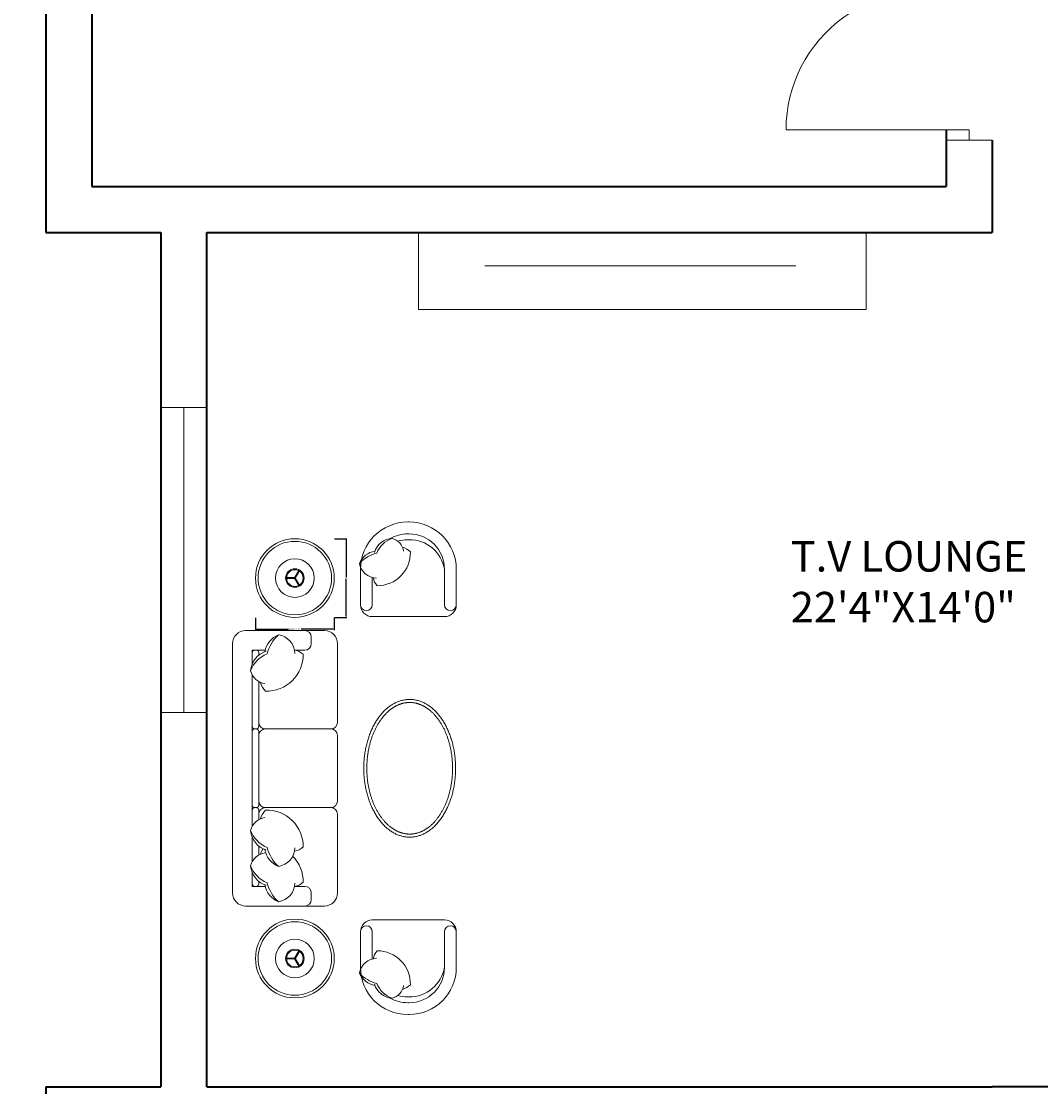
# Model space of a CAD drawing. Units: inches. Extents: x 1824 to 3509, y 619 to 2294.
# Tile 4 of 12: x 2001 to 2202, y 1115 to 1325. Entities that reach past the tile are written whole.
import ezdxf

# ---------------------------------------------------------------- set-up
doc = ezdxf.new("R2010")
doc.units = ezdxf.units.IN
for name, color, linetype, lineweight in [('A-ANNO-DIMS', 2, 'Continuous', 18), ('A-AREA-IDEN', 7, 'Continuous', 18), ('A-DOOR', 3, 'Continuous', 18), ('A-FURN', 8, 'Continuous', 13), ('A-GLAZ', 4, 'Continuous', 18), ('A-WALL', 7, 'Continuous', 35)]:
    doc.layers.add(name, color=color, linetype=linetype, lineweight=lineweight)
doc.styles.get("Standard").update_dxf_attribs({"font": 'arial.ttf'})
doc.dimstyles.get("Standard").update_dxf_attribs({"dimtxt": 0.18, "dimasz": 0.18, "dimexe": 0.18, "dimexo": 0.0625, "dimgap": 0.09, "dimtad": 0, "dimtih": 1, "dimtoh": 1, "dimdec": 4, "dimzin": 0, "dimdsep": 46, "dimtxsty": 'Standard', "dimcen": 0.09, "dimadec": 0, "dimazin": 0, "dimtfac": 1, "dimtdec": 4, "dimtofl": 0, "dimtmove": 0, "dimatfit": 3, "dimfxl": 1, "dimtolj": 1, "dimtzin": 0, "dimarcsym": 0})

# ---------------------------------------------------------------- blocks, each defined once
blk = doc.blocks.new('DOOR-BED-W-36')
for p, q in [((31.5, 29.8), (40.5, 29.8)), ((40.5, 29.8), (36, 29.8)), ((36, 29.8), (36, 27.8)), ((36, 2), (0, 2)), ((31.5, 0), (31.5, 0)), ((31.5, 0), (40.5, 0)), ((36, 0), (36, 2)), ((40.5, 0), (36, 0)), ((36, 0), (36, 0)), ((40.5, 0), (40.5, 0))]:
    blk.add_line(p, q)
blk.add_arc((27.25, 2), 27.25, 71.2585, 180)
blk = doc.blocks.new('WIN-60-SIDE')
for p, q in [((9, 60), (0, 60)), ((0, 60), (4.5, 60)), ((4.5, 60), (4.5, 0)), ((4.5, 0), (0, 0)), ((0, 0), (9, 0))]:
    blk.add_line(p, q)
blk = doc.blocks.new('LOUNGE-END-TABLE')
at = {"ltscale": 0.03}
for p, q in [((7.67, 7.78), (8.58, 9.36)), ((7.81, 7.7), (8.72, 9.27)), ((7.74, 7.82), (5.92, 7.82)), ((7.74, 7.66), (5.92, 7.66)), ((7.67, 7.7), (8.58, 6.12)), ((7.81, 7.78), (8.72, 6.21))]:
    blk.add_line(p, q, dxfattribs=at)
for radius in [7.74, 3.8, 1.82, 1.63]:
    blk.add_circle((7.74, 7.74), radius, dxfattribs=at)
blk.add_circle((7.74, 7.74), 7.22)
blk = doc.blocks.new('*D88')
at = {"layer": 'A-ANNO-DIMS', "color": 0, "lineweight": -2, "transparency": 16777216}
for p, q in [((2047.29, 1207.32), (2047.29, 1204.89)), ((2062.77, 1207.32), (2062.77, 1204.89)), ((2047.47, 1205.07), (2053.77, 1205.07)), ((2062.59, 1205.07), (2056.29, 1205.07))]:
    blk.add_line(p, q, dxfattribs=at)
at = {"layer": 'A-ANNO-DIMS', "color": 0, "transparency": 16777216}
for points in [[(2047.47, 1205.1), (2047.47, 1205.04), (2047.29, 1205.07)], [(2062.59, 1205.1), (2062.59, 1205.04), (2062.77, 1205.07)]]:
    blk.add_solid(points, dxfattribs=at)
at = {"layer": 'Defpoints', "color": 0, "transparency": 16777216}
for p in [(2047.29, 1207.39), (2062.77, 1207.39), (2062.77, 1205.07)]:
    blk.add_point(p, dxfattribs=at)
at = {"layer": 'A-ANNO-DIMS', "color": 0, "transparency": 16777216, "insert": (2055.03, 1205.07), "char_height": 0.18, "attachment_point": 5}
blk.add_mtext('\\A1;END TABLE 15 TYP.', dxfattribs=at)
blk = doc.blocks.new('*D89')
at = {"layer": 'A-ANNO-DIMS', "color": 0, "lineweight": -2, "transparency": 16777216}
for p, q in [((2062.83, 1222.87), (2065.27, 1222.87)), ((2065.09, 1222.69), (2065.09, 1215.31)), ((2065.09, 1207.57), (2065.09, 1214.95)), ((2062.83, 1207.39), (2065.27, 1207.39))]:
    blk.add_line(p, q, dxfattribs=at)
at = {"layer": 'A-ANNO-DIMS', "color": 0, "transparency": 16777216}
for points in [[(2065.06, 1222.69), (2065.12, 1222.69), (2065.09, 1222.87)], [(2065.06, 1207.57), (2065.12, 1207.57), (2065.09, 1207.39)]]:
    blk.add_solid(points, dxfattribs=at)
at = {"layer": 'Defpoints', "color": 0, "transparency": 16777216}
for p in [(2062.77, 1222.87), (2065.09, 1222.87), (2062.77, 1207.39)]:
    blk.add_point(p, dxfattribs=at)
at = {"layer": 'A-ANNO-DIMS', "color": 0, "transparency": 16777216, "insert": (2065.09, 1215.13), "char_height": 0.18, "attachment_point": 5}
blk.add_mtext('\\A1;15 TYP.', dxfattribs=at)
blk = doc.blocks.new('*D94')
at = {"layer": 'A-ANNO-DIMS', "color": 0, "lineweight": -2, "transparency": 16777216}
for p, q in [((1949.09, 1049.16), (1949.09, 1668.03)), ((1949.27, 1667.85), (2235.8, 1667.85)), ((2522.91, 1667.85), (2236.38, 1667.85)), ((2523.09, 1622.16), (2523.09, 1668.03))]:
    blk.add_line(p, q, dxfattribs=at)
at = {"layer": 'A-ANNO-DIMS', "color": 0, "transparency": 16777216}
for points in [[(1949.27, 1667.88), (1949.27, 1667.82), (1949.09, 1667.85)], [(2522.91, 1667.88), (2522.91, 1667.82), (2523.09, 1667.85)]]:
    blk.add_solid(points, dxfattribs=at)
at = {"layer": 'Defpoints', "color": 0, "transparency": 16777216}
for p in [(2523.09, 1667.85), (2523.09, 1622.1), (1949.09, 1049.1)]:
    blk.add_point(p, dxfattribs=at)
at = {"layer": 'A-ANNO-DIMS', "color": 0, "transparency": 16777216, "insert": (2236.09, 1667.85), "char_height": 0.18, "attachment_point": 5}
blk.add_mtext('\\A1;574', dxfattribs=at)
blk = doc.blocks.new('*D95')
at = {"layer": 'A-ANNO-DIMS', "color": 0, "lineweight": -2, "transparency": 16777216}
for p, q in [((2006.03, 1622.1), (1903.16, 1622.1)), ((1903.34, 1621.92), (1903.34, 1202.28)), ((1903.34, 782.28), (1903.34, 1201.92)), ((1949.03, 782.1), (1903.16, 782.1))]:
    blk.add_line(p, q, dxfattribs=at)
at = {"layer": 'A-ANNO-DIMS', "color": 0, "transparency": 16777216}
for points in [[(1903.31, 1621.92), (1903.37, 1621.92), (1903.34, 1622.1)], [(1903.31, 782.28), (1903.37, 782.28), (1903.34, 782.1)]]:
    blk.add_solid(points, dxfattribs=at)
at = {"layer": 'Defpoints', "color": 0, "transparency": 16777216}
for p in [(1903.34, 1622.1), (2006.09, 1622.1), (1949.09, 782.1)]:
    blk.add_point(p, dxfattribs=at)
at = {"layer": 'A-ANNO-DIMS', "color": 0, "transparency": 16777216, "insert": (1903.34, 1202.1), "char_height": 0.18, "attachment_point": 5}
blk.add_mtext('\\A1;840', dxfattribs=at)

msp = doc.modelspace()

# ---------------------------------------------------------------- linework, layer by layer
at = {"layer": 'A-FURN'}
msp.add_line((2092.3975, 1276.5357), (2153.4936, 1276.5357), dxfattribs=at)
msp.add_lwpolyline([(2079.3103, 1283.1012), (2167.3585, 1283.1012), (2167.3585, 1267.9224), (2079.3103, 1267.9224)], close=True, dxfattribs=at)
at = {"layer": 'A-FURN', "ltscale": 0.03}
for points in [[(2077.3473, 1207.5438), (2084.4419, 1207.5438, 0.41421356), (2086.768, 1209.8699), (2086.768, 1216.8482, 0.41421356), (2077.4636, 1226.1526), (2077.3473, 1226.1526), (2077.231, 1226.1526, 0.41421356), (2067.9266, 1216.8482), (2067.9266, 1209.8699, 0.41421356), (2070.2527, 1207.5438), (2077.3473, 1207.5438)], [(2077.3473, 1147.8942), (2084.4419, 1147.8942, -0.41421356), (2086.768, 1145.5681), (2086.768, 1138.5898, -0.41421356), (2077.4636, 1129.2854), (2077.3473, 1129.2854), (2077.231, 1129.2854, -0.41421356), (2067.9266, 1138.5898), (2067.9266, 1145.5681, -0.41421356), (2070.2527, 1147.8942), (2077.3473, 1147.8942)]]:
    msp.add_lwpolyline(points, format="xyb", dxfattribs=at)
at = {"layer": 'A-FURN'}
for points in [[(2073.7671, 1222.9061, -0.13059149), (2077.231, 1223.8265), (2077.3473, 1223.8265)], [(2084.4419, 1216.8482, 0.41421356), (2077.4636, 1223.8265), (2077.3473, 1223.8265)], [(2067.7364, 1218.0222, -0.14772988), (2071.1356, 1220.0211, -0.21334276), (2074.135, 1222.9527, -0.17866181)], [(2070.666, 1220.1804, -0.30666349), (2074.135, 1222.9527, -0.30632997), (2076.4012, 1220.4208, 0.87284716)], [(2075.2481, 1222.4128, -0.07238424), (2077.231, 1222.6634), (2077.3473, 1222.6634)], [(2084.4419, 1216.8482, 0.37271891), (2077.4636, 1222.6634), (2077.3473, 1222.6634)], [(2071.069, 1215.0906, -0.35677236), (2067.7364, 1218.0222, -0.24954205), (2070.756, 1220.4381, 9.61688035)], [(2070.4828, 1215.1615, 0.16554063), (2071.2023, 1213.6248, 0.42598917), (2077.7342, 1220.2876, 0.12152332), (2076.1837, 1221.2059, -7.11546429)], [(2070.2527, 1215.2175), (2070.2527, 1209.8699, -0.41421356), (2069.0897, 1208.7068), (2069.0897, 1208.7068, -0.41421356), (2067.9266, 1209.8699)], [(2084.4419, 1216.8483), (2084.4419, 1209.8699, 0.41421356), (2085.605, 1208.7068), (2085.605, 1208.7068, 0.41421356), (2086.768, 1209.8699)], [(2056.9664, 1204.8075, -0.41421356), (2058.2564, 1203.5176), (2058.2564, 1202.2276, -0.41421356), (2056.9664, 1200.9377), (2054.9679, 1200.9377)], [(2051.7945, 1203.9865, 0.14772988), (2049.5776, 1200.2164, 0.21334276), (2046.3262, 1196.8899, 0.17866181)], [(2055.0459, 1200.2904, 0.35677236), (2051.7945, 1203.9865, 0.24954205), (2049.1151, 1200.6375, -9.61688035)], [(2049.401, 1200.7373, 0.30666349), (2046.3262, 1196.8899, 0.30632997), (2049.1343, 1194.3765, -0.87284716)], [(2047.9369, 1199.9533), (2047.9369, 1200.4217, 0.41421356), (2047.421, 1200.9377), (2047.163, 1200.9377, 0.41421356), (2046.647, 1200.4217)], [(2054.9673, 1200.9405, -0.16554063), (2056.6716, 1200.1425, -0.42598917), (2049.2821, 1192.898, -0.12152332), (2048.2635, 1194.6177, 7.11546429)], [(2046.647, 1200.4217), (2046.647, 1198.2241, 0.41421356)], [(2046.647, 1196.0781), (2046.647, 1185.9745, 0.41421356), (2047.163, 1185.4586), (2047.421, 1185.4586, 0.41421356), (2047.9369, 1185.9745), (2047.9369, 1194.7792, 0.41421356)], [(2047.9369, 1186.7485, 0.41421356), (2049.2269, 1185.4586), (2062.1262, 1185.4586, 0.41421356)], [(2047.9369, 1184.1686, -0.41421356), (2049.2269, 1185.4586)], [(2047.9369, 1171.2693, 0.41421356), (2049.2269, 1169.9794)], [(2046.647, 1166.3087), (2046.647, 1169.4634, -0.41421356), (2047.163, 1169.9794), (2047.421, 1169.9794, -0.41421356), (2047.9369, 1169.4634), (2047.9369, 1167.6076, -0.41421356)], [(2047.9369, 1168.6895, -0.41421356), (2049.2269, 1169.9794), (2062.1262, 1169.9794, -0.41421356)], [(2054.9673, 1161.4463, 0.16554063), (2056.6716, 1162.2442, 0.42598917), (2049.2821, 1169.4887, 0.12152332), (2048.2635, 1167.769, -7.11546429)], [(2049.401, 1161.6495, -0.30666349), (2046.3262, 1165.4969, -0.30632997), (2049.1343, 1168.0103, 0.87284716)], [(2051.7945, 1158.4002, -0.14772988), (2049.5776, 1162.1703, -0.21334276), (2046.3262, 1165.4969, -0.17866181)], [(2046.647, 1159.3599), (2046.647, 1164.1627, -0.41421356)], [(2049.401, 1154.7007, -0.30666349), (2046.3262, 1158.5481, -0.30632997), (2049.1343, 1161.0615, 0.87284716)], [(2047.9369, 1162.4334), (2047.9369, 1160.6588, -0.41421356)], [(2048.7678, 1161.9017, 0.07186538), (2048.2635, 1160.8202, -7.11546429)], [(2055.0459, 1162.0964, -0.35677236), (2051.7945, 1158.4002, -0.24954205), (2049.1151, 1161.7493, 9.61688035)], [(2054.9673, 1154.4975, 0.16554063), (2056.6716, 1155.2954, 0.20023115), (2054.5959, 1160.416, 0.12152332)], [(2051.7945, 1151.4514, -0.14772988), (2049.5776, 1155.2215, -0.21334276), (2046.3262, 1158.5481, -0.17866181)], [(2046.647, 1157.2139), (2046.647, 1154.5003), (2049.182, 1154.5003, -0.41421356)], [(2046.647, 1155.0162), (2046.647, 1157.2139, -0.41421356)], [(2047.9369, 1155.4846), (2047.9369, 1155.0162, -0.41421356), (2047.421, 1154.5003), (2047.163, 1154.5003, -0.41421356), (2046.647, 1155.0162)], [(2055.0459, 1155.1476, -0.35677236), (2051.7945, 1151.4514, -0.24954205), (2049.1151, 1154.8005, 9.61688035)], [(2054.9679, 1154.5003), (2056.9664, 1154.5003, -0.41421356), (2058.2564, 1153.2103), (2058.2564, 1151.9204, -0.41421356), (2056.9664, 1150.6305)], [(2070.2527, 1140.2205), (2070.2527, 1145.5681, 0.41421356), (2069.0897, 1146.7311), (2069.0897, 1146.7311, 0.41421356), (2067.9266, 1145.5681)], [(2084.4419, 1138.5897), (2084.4419, 1145.5681, -0.41421356), (2085.605, 1146.7311), (2085.605, 1146.7311, -0.41421356), (2086.768, 1145.5681)], [(2071.069, 1140.3473, 0.35677236), (2067.7364, 1137.4157, 0.24954205), (2070.756, 1134.9998, -9.61688035)], [(2070.4828, 1140.2764, -0.16554063), (2071.2023, 1141.8131, -0.42598917), (2077.7342, 1135.1504, -0.12152332), (2076.1837, 1134.2321, 7.11546429)], [(2084.4419, 1138.5898, -0.37271891), (2077.4636, 1132.7745), (2077.3473, 1132.7745)], [(2084.4419, 1138.5898, -0.41421356), (2077.4636, 1131.6115), (2077.3473, 1131.6115)], [(2067.7364, 1137.4157, 0.14772988), (2071.1356, 1135.4169, 0.21334276), (2074.135, 1132.4853, 0.17866181)], [(2070.666, 1135.2576, 0.30666349), (2074.135, 1132.4853, 0.30632997), (2076.4012, 1135.0171, -0.87284716)], [(2073.7671, 1132.5319, 0.13059149), (2077.231, 1131.6115), (2077.3473, 1131.6115)], [(2075.2481, 1133.0251, 0.07238424), (2077.231, 1132.7745), (2077.3473, 1132.7745)]]:
    msp.add_lwpolyline(points, format="xyb", dxfattribs=at)
at = {"layer": 'A-FURN', "ltscale": 0.03}
msp.add_lwpolyline([(2060.8362, 1204.8075, -0.41421356), (2063.4161, 1202.2276), (2063.4161, 1186.7485, -0.41421356), (2062.1262, 1185.4586, -0.41421356), (2063.4161, 1184.1686), (2063.4161, 1171.2693, -0.41421356), (2062.1262, 1169.9794, -0.41421356), (2063.4161, 1168.6895), (2063.4161, 1153.2103, -0.41421356), (2060.8362, 1150.6305), (2045.3571, 1150.6305, -0.41421356), (2042.7772, 1153.2103), (2042.7772, 1202.2276, -0.41421356), (2045.3571, 1204.8075)], format="xyb", close=True, dxfattribs=at)
at = {"layer": 'A-FURN'}
for points in [[(2049.182, 1200.9377), (2046.647, 1200.9377), (2046.647, 1198.2241)], [(2046.647, 1196.0781), (2046.647, 1166.3087)], [(2046.647, 1164.1627), (2046.647, 1159.3599)]]:
    msp.add_lwpolyline(points, dxfattribs=at)
msp.add_lwpolyline([(2046.647, 1170.4954), (2046.647, 1184.9426, -0.41421356), (2047.163, 1185.4586), (2047.421, 1185.4586, -0.41421356), (2047.9369, 1184.9426), (2047.9369, 1170.4954, -0.41421356), (2047.421, 1169.9794), (2047.163, 1169.9794, -0.41421356)], format="xyb", close=True, dxfattribs=at)
at = {"layer": 'A-FURN', "ltscale": 0.03}
msp.add_polyline3d([(2077.6053, 1191.2632, 0), (2077.4344, 1191.2608, 0), (2077.2636, 1191.2535, 0), (2077.0929, 1191.2414, 0), (2076.9224, 1191.2244, 0), (2076.7521, 1191.2026, 0), (2076.5822, 1191.176, 0), (2076.4126, 1191.1446, 0), (2076.2434, 1191.1083, 0), (2076.0748, 1191.0672, 0), (2075.9066, 1191.0214, 0), (2075.7391, 1190.9708, 0), (2075.5723, 1190.9155, 0), (2075.4061, 1190.8554, 0), (2075.2408, 1190.7906, 0), (2075.0763, 1190.7211, 0), (2074.9127, 1190.647, 0), (2074.7501, 1190.5683, 0), (2074.5885, 1190.4849, 0), (2074.428, 1190.397, 0), (2074.2686, 1190.3046, 0), (2074.1104, 1190.2076, 0), (2073.9535, 1190.1061, 0), (2073.7979, 1190.0003, 0), (2073.6436, 1189.89, 0), (2073.4908, 1189.7753, 0), (2073.3394, 1189.6564, 0), (2073.1896, 1189.5332, 0), (2073.0413, 1189.4057, 0), (2072.8947, 1189.2741, 0), (2072.7497, 1189.1383, 0), (2072.6066, 1188.9984, 0), (2072.4651, 1188.8545, 0), (2072.3256, 1188.7066, 0), (2072.1879, 1188.5547, 0), (2072.0522, 1188.399, 0), (2071.9184, 1188.2395, 0), (2071.7867, 1188.0762, 0), (2071.6571, 1187.9091, 0), (2071.5296, 1187.7385, 0), (2071.4043, 1187.5642, 0), (2071.2812, 1187.3864, 0), (2071.1603, 1187.2052, 0), (2071.0418, 1187.0205, 0), (2070.9256, 1186.8325, 0), (2070.8119, 1186.6413, 0), (2070.7005, 1186.4469, 0), (2070.5916, 1186.2493, 0), (2070.4853, 1186.0487, 0), (2070.3815, 1185.8451, 0), (2070.2802, 1185.6386, 0), (2070.1816, 1185.4292, 0), (2070.0857, 1185.2171, 0), (2069.9924, 1185.0023, 0), (2069.9019, 1184.7849, 0), (2069.8142, 1184.565, 0), (2069.7292, 1184.3426, 0), (2069.647, 1184.1178, 0), (2069.5677, 1183.8908, 0), (2069.4913, 1183.6615, 0), (2069.4178, 1183.4301, 0), (2069.3472, 1183.1967, 0), (2069.2796, 1182.9613, 0), (2069.2149, 1182.724, 0), (2069.1533, 1182.485, 0), (2069.0947, 1182.2442, 0), (2069.0391, 1182.0018, 0), (2068.9866, 1181.7579, 0), (2068.9372, 1181.5125, 0), (2068.8909, 1181.2657, 0), (2068.8477, 1181.0177, 0), (2068.8076, 1180.7686, 0), (2068.7708, 1180.5183, 0), (2068.737, 1180.267, 0), (2068.7065, 1180.0148, 0), (2068.6791, 1179.7618, 0), (2068.6549, 1179.508, 0), (2068.6339, 1179.2537, 0), (2068.6162, 1178.9987, 0), (2068.6017, 1178.7433, 0), (2068.5903, 1178.4876, 0), (2068.5823, 1178.2315, 0), (2068.5774, 1177.9753, 0), (2068.5758, 1177.719, 0), (2068.5774, 1177.4627, 0), (2068.5823, 1177.2064, 0), (2068.5903, 1176.9504, 0), (2068.6017, 1176.6946, 0), (2068.6162, 1176.4393, 0), (2068.6339, 1176.1843, 0), (2068.6549, 1175.9299, 0), (2068.6791, 1175.6762, 0), (2068.7065, 1175.4232, 0), (2068.737, 1175.171, 0), (2068.7708, 1174.9197, 0), (2068.8076, 1174.6694, 0), (2068.8477, 1174.4202, 0), (2068.8909, 1174.1722, 0), (2068.9372, 1173.9255, 0), (2068.9866, 1173.6801, 0), (2069.0391, 1173.4362, 0), (2069.0947, 1173.1938, 0), (2069.1533, 1172.953, 0), (2069.2149, 1172.714, 0), (2069.2796, 1172.4767, 0), (2069.3472, 1172.2413, 0), (2069.4178, 1172.0078, 0), (2069.4913, 1171.7765, 0), (2069.5677, 1171.5472, 0), (2069.647, 1171.3201, 0), (2069.7292, 1171.0954, 0), (2069.8142, 1170.873, 0), (2069.9019, 1170.6531, 0), (2069.9924, 1170.4357, 0), (2070.0857, 1170.2209, 0), (2070.1816, 1170.0088, 0), (2070.2802, 1169.7994, 0), (2070.3815, 1169.5929, 0), (2070.4853, 1169.3893, 0), (2070.5916, 1169.1887, 0), (2070.7005, 1168.9911, 0), (2070.8119, 1168.7967, 0), (2070.9256, 1168.6054, 0), (2071.0418, 1168.4174, 0), (2071.1603, 1168.2328, 0), (2071.2812, 1168.0516, 0), (2071.4043, 1167.8738, 0), (2071.5296, 1167.6995, 0), (2071.6571, 1167.5288, 0), (2071.7867, 1167.3618, 0), (2071.9184, 1167.1985, 0), (2072.0522, 1167.039, 0), (2072.1879, 1166.8832, 0), (2072.3256, 1166.7314, 0), (2072.4651, 1166.5835, 0), (2072.6066, 1166.4396, 0), (2072.7497, 1166.2997, 0), (2072.8947, 1166.1639, 0), (2073.0413, 1166.0323, 0), (2073.1896, 1165.9048, 0), (2073.3394, 1165.7816, 0), (2073.4908, 1165.6626, 0), (2073.6436, 1165.548, 0), (2073.7979, 1165.4377, 0), (2073.9535, 1165.3318, 0), (2074.1104, 1165.2304, 0), (2074.2686, 1165.1334, 0), (2074.428, 1165.041, 0), (2074.5885, 1164.953, 0), (2074.7501, 1164.8697, 0), (2074.9127, 1164.7909, 0), (2075.0763, 1164.7168, 0), (2075.2408, 1164.6474, 0), (2075.4061, 1164.5826, 0), (2075.5723, 1164.5225, 0), (2075.7391, 1164.4672, 0), (2075.9066, 1164.4166, 0), (2076.0748, 1164.3707, 0), (2076.2434, 1164.3297, 0), (2076.4126, 1164.2934, 0), (2076.5822, 1164.262, 0), (2076.7521, 1164.2353, 0), (2076.9224, 1164.2135, 0), (2077.0929, 1164.1966, 0), (2077.2636, 1164.1844, 0), (2077.4344, 1164.1772, 0), (2077.6053, 1164.1747, 0), (2077.7762, 1164.1772, 0), (2077.947, 1164.1844, 0), (2078.1177, 1164.1966, 0), (2078.2882, 1164.2135, 0), (2078.4585, 1164.2353, 0), (2078.6284, 1164.262, 0), (2078.798, 1164.2934, 0), (2078.9672, 1164.3297, 0), (2079.1358, 1164.3707, 0), (2079.304, 1164.4166, 0), (2079.4715, 1164.4672, 0), (2079.6383, 1164.5225, 0), (2079.8045, 1164.5826, 0), (2079.9698, 1164.6474, 0), (2080.1343, 1164.7168, 0), (2080.2979, 1164.7909, 0), (2080.4605, 1164.8697, 0), (2080.6221, 1164.953, 0), (2080.7826, 1165.041, 0), (2080.942, 1165.1334, 0), (2081.1002, 1165.2304, 0), (2081.2571, 1165.3318, 0), (2081.4127, 1165.4377, 0), (2081.567, 1165.548, 0), (2081.7198, 1165.6626, 0), (2081.8712, 1165.7816, 0), (2082.021, 1165.9048, 0), (2082.1693, 1166.0323, 0), (2082.3159, 1166.1639, 0), (2082.4609, 1166.2997, 0), (2082.604, 1166.4396, 0), (2082.7455, 1166.5835, 0), (2082.885, 1166.7314, 0), (2083.0227, 1166.8832, 0), (2083.1584, 1167.039, 0), (2083.2922, 1167.1985, 0), (2083.4239, 1167.3618, 0), (2083.5535, 1167.5288, 0), (2083.681, 1167.6995, 0), (2083.8063, 1167.8738, 0), (2083.9294, 1168.0516, 0), (2084.0503, 1168.2328, 0), (2084.1688, 1168.4174, 0), (2084.285, 1168.6054, 0), (2084.3987, 1168.7967, 0), (2084.5101, 1168.9911, 0), (2084.619, 1169.1887, 0), (2084.7253, 1169.3893, 0), (2084.8291, 1169.5929, 0), (2084.9304, 1169.7994, 0), (2085.029, 1170.0088, 0), (2085.1249, 1170.2209, 0), (2085.2182, 1170.4357, 0), (2085.3087, 1170.6531, 0), (2085.3964, 1170.873, 0), (2085.4814, 1171.0954, 0), (2085.5636, 1171.3201, 0), (2085.6429, 1171.5472, 0), (2085.7193, 1171.7765, 0), (2085.7928, 1172.0078, 0), (2085.8634, 1172.2413, 0), (2085.931, 1172.4767, 0), (2085.9957, 1172.714, 0), (2086.0573, 1172.953, 0), (2086.1159, 1173.1938, 0), (2086.1715, 1173.4362, 0), (2086.224, 1173.6801, 0), (2086.2734, 1173.9255, 0), (2086.3197, 1174.1722, 0), (2086.3629, 1174.4202, 0), (2086.403, 1174.6694, 0), (2086.4398, 1174.9197, 0), (2086.4736, 1175.171, 0), (2086.5041, 1175.4232, 0), (2086.5315, 1175.6762, 0), (2086.5557, 1175.9299, 0), (2086.5767, 1176.1843, 0), (2086.5944, 1176.4393, 0), (2086.6089, 1176.6946, 0), (2086.6203, 1176.9504, 0), (2086.6283, 1177.2064, 0), (2086.6332, 1177.4627, 0), (2086.6348, 1177.719, 0), (2086.6332, 1177.9753, 0), (2086.6283, 1178.2315, 0), (2086.6203, 1178.4876, 0), (2086.6089, 1178.7433, 0), (2086.5944, 1178.9987, 0), (2086.5767, 1179.2537, 0), (2086.5557, 1179.508, 0), (2086.5315, 1179.7618, 0), (2086.5041, 1180.0148, 0), (2086.4736, 1180.267, 0), (2086.4398, 1180.5183, 0), (2086.403, 1180.7686, 0), (2086.3629, 1181.0177, 0), (2086.3197, 1181.2657, 0), (2086.2734, 1181.5125, 0), (2086.224, 1181.7579, 0), (2086.1715, 1182.0018, 0), (2086.1159, 1182.2442, 0), (2086.0573, 1182.485, 0), (2085.9957, 1182.724, 0), (2085.931, 1182.9613, 0), (2085.8634, 1183.1967, 0), (2085.7928, 1183.4301, 0), (2085.7193, 1183.6615, 0), (2085.6429, 1183.8908, 0), (2085.5636, 1184.1178, 0), (2085.4814, 1184.3426, 0), (2085.3964, 1184.565, 0), (2085.3087, 1184.7849, 0), (2085.2182, 1185.0023, 0), (2085.1249, 1185.2171, 0), (2085.029, 1185.4292, 0), (2084.9304, 1185.6386, 0), (2084.8291, 1185.8451, 0), (2084.7253, 1186.0487, 0), (2084.619, 1186.2493, 0), (2084.5101, 1186.4469, 0), (2084.3987, 1186.6413, 0), (2084.285, 1186.8325, 0), (2084.1688, 1187.0205, 0), (2084.0503, 1187.2052, 0), (2083.9294, 1187.3864, 0), (2083.8063, 1187.5642, 0), (2083.681, 1187.7385, 0), (2083.5535, 1187.9091, 0), (2083.4239, 1188.0762, 0), (2083.2922, 1188.2395, 0), (2083.1584, 1188.399, 0), (2083.0227, 1188.5547, 0), (2082.885, 1188.7066, 0), (2082.7455, 1188.8545, 0), (2082.604, 1188.9984, 0), (2082.4609, 1189.1383, 0), (2082.3159, 1189.2741, 0), (2082.1693, 1189.4057, 0), (2082.021, 1189.5332, 0), (2081.8712, 1189.6564, 0), (2081.7198, 1189.7753, 0), (2081.567, 1189.89, 0), (2081.4127, 1190.0003, 0), (2081.2571, 1190.1061, 0), (2081.1002, 1190.2076, 0), (2080.942, 1190.3046, 0), (2080.7826, 1190.397, 0), (2080.6221, 1190.4849, 0), (2080.4605, 1190.5683, 0), (2080.2979, 1190.647, 0), (2080.1343, 1190.7211, 0), (2079.9698, 1190.7906, 0), (2079.8045, 1190.8554, 0), (2079.6383, 1190.9155, 0), (2079.4715, 1190.9708, 0), (2079.304, 1191.0214, 0), (2079.1358, 1191.0672, 0), (2078.9672, 1191.1083, 0), (2078.798, 1191.1446, 0), (2078.6284, 1191.176, 0), (2078.4585, 1191.2026, 0), (2078.2882, 1191.2244, 0), (2078.1177, 1191.2414, 0), (2077.947, 1191.2535, 0), (2077.7762, 1191.2608, 0), (2077.6053, 1191.2632, 0)], dxfattribs=at)
at = {"layer": 'A-FURN'}
msp.add_polyline3d([(2077.6053, 1190.6613, 0), (2077.513, 1190.6605, 0), (2077.4202, 1190.6581, 0), (2077.327, 1190.6541, 0), (2077.2334, 1190.6485, 0), (2077.1394, 1190.6412, 0), (2077.0451, 1190.6323, 0), (2076.9504, 1190.6216, 0), (2076.8553, 1190.6092, 0), (2076.7599, 1190.5951, 0), (2076.6642, 1190.5793, 0), (2076.5682, 1190.5616, 0), (2076.4719, 1190.5422, 0), (2076.3753, 1190.5209, 0), (2076.2784, 1190.4978, 0), (2076.1812, 1190.4728, 0), (2076.0839, 1190.446, 0), (2075.9862, 1190.4172, 0), (2075.8884, 1190.3865, 0), (2075.7904, 1190.3539, 0), (2075.6921, 1190.3193, 0), (2075.5937, 1190.2827, 0), (2075.4951, 1190.2441, 0), (2075.3964, 1190.2034, 0), (2075.2977, 1190.1607, 0), (2075.1988, 1190.116, 0), (2075.0999, 1190.0692, 0), (2075.001, 1190.0203, 0), (2074.9022, 1189.9694, 0), (2074.8034, 1189.9164, 0), (2074.7047, 1189.8614, 0), (2074.606, 1189.8043, 0), (2074.5076, 1189.7451, 0), (2074.4093, 1189.6838, 0), (2074.3112, 1189.6205, 0), (2074.2133, 1189.5551, 0), (2074.1157, 1189.4876, 0), (2074.0184, 1189.418, 0), (2073.9214, 1189.3464, 0), (2073.8248, 1189.2726, 0), (2073.7285, 1189.1968, 0), (2073.6327, 1189.1188, 0), (2073.5372, 1189.0388, 0), (2073.4423, 1188.9565, 0), (2073.3478, 1188.8719, 0), (2073.2538, 1188.7851, 0), (2073.1604, 1188.6962, 0), (2073.0675, 1188.6051, 0), (2072.9752, 1188.5119, 0), (2072.8835, 1188.4165, 0), (2072.7924, 1188.3192, 0), (2072.702, 1188.2197, 0), (2072.6123, 1188.1183, 0), (2072.5232, 1188.015, 0), (2072.4349, 1187.9097, 0), (2072.3474, 1187.8025, 0), (2072.2606, 1187.6934, 0), (2072.1746, 1187.5825, 0), (2072.0895, 1187.4698, 0), (2072.0052, 1187.3553, 0), (2071.9218, 1187.239, 0), (2071.8393, 1187.1211, 0), (2071.7577, 1187.0015, 0), (2071.6771, 1186.8802, 0), (2071.5974, 1186.7573, 0), (2071.5188, 1186.6328, 0), (2071.4412, 1186.5067, 0), (2071.3646, 1186.3792, 0), (2071.2891, 1186.2501, 0), (2071.2147, 1186.1196, 0), (2071.1414, 1185.9877, 0), (2071.0693, 1185.8543, 0), (2070.9983, 1185.7196, 0), (2070.9286, 1185.5836, 0), (2070.86, 1185.4462, 0), (2070.7928, 1185.3076, 0), (2070.7267, 1185.1677, 0), (2070.662, 1185.0267, 0), (2070.5986, 1184.8844, 0), (2070.5366, 1184.741, 0), (2070.4759, 1184.5965, 0), (2070.4166, 1184.4509, 0), (2070.3588, 1184.3043, 0), (2070.3023, 1184.1566, 0), (2070.2474, 1184.0082, 0), (2070.1939, 1183.8593, 0), (2070.1419, 1183.71, 0), (2070.0913, 1183.5603, 0), (2070.0421, 1183.4103, 0), (2069.9944, 1183.2598, 0), (2069.9481, 1183.109, 0), (2069.9032, 1182.9578, 0), (2069.8597, 1182.8063, 0), (2069.8177, 1182.6545, 0), (2069.777, 1182.5023, 0), (2069.7378, 1182.3498, 0), (2069.6999, 1182.197, 0), (2069.6634, 1182.0439, 0), (2069.6283, 1181.8906, 0), (2069.5945, 1181.7369, 0), (2069.5622, 1181.583, 0), (2069.5311, 1181.4289, 0), (2069.5015, 1181.2745, 0), (2069.4731, 1181.1198, 0), (2069.4462, 1180.965, 0), (2069.4205, 1180.8099, 0), (2069.3962, 1180.6546, 0), (2069.3732, 1180.4992, 0), (2069.3515, 1180.3435, 0), (2069.3311, 1180.1877, 0), (2069.312, 1180.0317, 0), (2069.2942, 1179.8756, 0), (2069.2777, 1179.7193, 0), (2069.2625, 1179.5629, 0), (2069.2486, 1179.4064, 0), (2069.2359, 1179.2498, 0), (2069.2245, 1179.0931, 0), (2069.2144, 1178.9362, 0), (2069.2055, 1178.7793, 0), (2069.1979, 1178.6224, 0), (2069.1915, 1178.4653, 0), (2069.1863, 1178.3083, 0), (2069.1823, 1178.1512, 0), (2069.1796, 1177.994, 0), (2069.1781, 1177.8369, 0), (2069.1778, 1177.6797, 0), (2069.1787, 1177.5225, 0), (2069.1808, 1177.3654, 0), (2069.1842, 1177.2082, 0), (2069.1887, 1177.0512, 0), (2069.1945, 1176.8941, 0), (2069.2015, 1176.7371, 0), (2069.2098, 1176.5802, 0), (2069.2193, 1176.4233, 0), (2069.2301, 1176.2665, 0), (2069.2421, 1176.1099, 0), (2069.2554, 1175.9533, 0), (2069.27, 1175.7968, 0), (2069.2858, 1175.6405, 0), (2069.303, 1175.4843, 0), (2069.3214, 1175.3282, 0), (2069.3411, 1175.1723, 0), (2069.3622, 1175.0166, 0), (2069.3845, 1174.861, 0), (2069.4082, 1174.7057, 0), (2069.4332, 1174.5505, 0), (2069.4595, 1174.3955, 0), (2069.4871, 1174.2408, 0), (2069.5161, 1174.0863, 0), (2069.5465, 1173.932, 0), (2069.5782, 1173.778, 0), (2069.6112, 1173.6242, 0), (2069.6457, 1173.4707, 0), (2069.6815, 1173.3174, 0), (2069.7186, 1173.1645, 0), (2069.7572, 1173.0119, 0), (2069.7972, 1172.8595, 0), (2069.8385, 1172.7075, 0), (2069.8813, 1172.5558, 0), (2069.9255, 1172.4045, 0), (2069.971, 1172.2535, 0), (2070.0181, 1172.1029, 0), (2070.0665, 1171.9526, 0), (2070.1164, 1171.8027, 0), (2070.1677, 1171.6533, 0), (2070.2205, 1171.5042, 0), (2070.2747, 1171.3555, 0), (2070.3304, 1171.2074, 0), (2070.3875, 1171.0602, 0), (2070.4461, 1170.9141, 0), (2070.5061, 1170.7691, 0), (2070.5674, 1170.6251, 0), (2070.6302, 1170.4823, 0), (2070.6942, 1170.3406, 0), (2070.7596, 1170.2001, 0), (2070.8262, 1170.0609, 0), (2070.8942, 1169.9229, 0), (2070.9633, 1169.7862, 0), (2071.0337, 1169.6508, 0), (2071.1052, 1169.5168, 0), (2071.1779, 1169.3842, 0), (2071.2518, 1169.2529, 0), (2071.3267, 1169.1231, 0), (2071.4027, 1168.9948, 0), (2071.4799, 1168.868, 0), (2071.558, 1168.7427, 0), (2071.6372, 1168.619, 0), (2071.7173, 1168.4969, 0), (2071.7984, 1168.3765, 0), (2071.8804, 1168.2577, 0), (2071.9634, 1168.1406, 0), (2072.0473, 1168.0252, 0), (2072.132, 1167.9116, 0), (2072.2175, 1167.7998, 0), (2072.3039, 1167.6898, 0), (2072.3911, 1167.5817, 0), (2072.479, 1167.4754, 0), (2072.5677, 1167.3711, 0), (2072.657, 1167.2687, 0), (2072.7471, 1167.1683, 0), (2072.8379, 1167.0699, 0), (2072.9293, 1166.9735, 0), (2073.0213, 1166.8792, 0), (2073.1139, 1166.7871, 0), (2073.207, 1166.697, 0), (2073.3007, 1166.6092, 0), (2073.395, 1166.5235, 0), (2073.4897, 1166.4401, 0), (2073.5849, 1166.3589, 0), (2073.6805, 1166.2799, 0), (2073.7766, 1166.203, 0), (2073.8731, 1166.1282, 0), (2073.9699, 1166.0555, 0), (2074.067, 1165.9849, 0), (2074.1645, 1165.9163, 0), (2074.2622, 1165.8499, 0), (2074.3602, 1165.7855, 0), (2074.4584, 1165.7232, 0), (2074.5568, 1165.663, 0), (2074.6553, 1165.6049, 0), (2074.754, 1165.5488, 0), (2074.8528, 1165.4948, 0), (2074.9516, 1165.4428, 0), (2075.0505, 1165.393, 0), (2075.1494, 1165.3451, 0), (2075.2482, 1165.2993, 0), (2075.3471, 1165.2556, 0), (2075.4458, 1165.2139, 0), (2075.5444, 1165.1743, 0), (2075.6429, 1165.1367, 0), (2075.7413, 1165.1011, 0), (2075.8394, 1165.0675, 0), (2075.9373, 1165.0358, 0), (2076.0351, 1165.0061, 0), (2076.1326, 1164.9783, 0), (2076.2298, 1164.9524, 0), (2076.3269, 1164.9284, 0), (2076.4236, 1164.9062, 0), (2076.5201, 1164.8858, 0), (2076.6162, 1164.8673, 0), (2076.7121, 1164.8505, 0), (2076.8077, 1164.8356, 0), (2076.9029, 1164.8223, 0), (2076.9978, 1164.8108, 0), (2077.0923, 1164.801, 0), (2077.1865, 1164.7929, 0), (2077.2803, 1164.7865, 0), (2077.3736, 1164.7817, 0), (2077.4666, 1164.7785, 0), (2077.5592, 1164.7769, 0), (2077.6514, 1164.7769, 0), (2077.744, 1164.7785, 0), (2077.837, 1164.7817, 0), (2077.9303, 1164.7865, 0), (2078.0241, 1164.7929, 0), (2078.1183, 1164.801, 0), (2078.2128, 1164.8108, 0), (2078.3077, 1164.8223, 0), (2078.4029, 1164.8356, 0), (2078.4985, 1164.8505, 0), (2078.5944, 1164.8673, 0), (2078.6905, 1164.8858, 0), (2078.787, 1164.9062, 0), (2078.8838, 1164.9284, 0), (2078.9808, 1164.9524, 0), (2079.078, 1164.9783, 0), (2079.1755, 1165.0061, 0), (2079.2733, 1165.0358, 0), (2079.3712, 1165.0675, 0), (2079.4693, 1165.1011, 0), (2079.5677, 1165.1367, 0), (2079.6662, 1165.1743, 0), (2079.7648, 1165.2139, 0), (2079.8635, 1165.2556, 0), (2079.9624, 1165.2993, 0), (2080.0612, 1165.3451, 0), (2080.1601, 1165.393, 0), (2080.259, 1165.4428, 0), (2080.3578, 1165.4948, 0), (2080.4566, 1165.5488, 0), (2080.5553, 1165.6049, 0), (2080.6538, 1165.663, 0), (2080.7522, 1165.7232, 0), (2080.8504, 1165.7855, 0), (2080.9484, 1165.8499, 0), (2081.0461, 1165.9163, 0), (2081.1436, 1165.9849, 0), (2081.2407, 1166.0555, 0), (2081.3375, 1166.1282, 0), (2081.434, 1166.203, 0), (2081.5301, 1166.2799, 0), (2081.6257, 1166.3589, 0), (2081.7209, 1166.4401, 0), (2081.8156, 1166.5235, 0), (2081.9099, 1166.6092, 0), (2082.0036, 1166.697, 0), (2082.0967, 1166.7871, 0), (2082.1893, 1166.8792, 0), (2082.2813, 1166.9735, 0), (2082.3727, 1167.0699, 0), (2082.4635, 1167.1683, 0), (2082.5536, 1167.2687, 0), (2082.6429, 1167.3711, 0), (2082.7316, 1167.4754, 0), (2082.8195, 1167.5817, 0), (2082.9067, 1167.6898, 0), (2082.9931, 1167.7998, 0), (2083.0786, 1167.9116, 0), (2083.1633, 1168.0252, 0), (2083.2472, 1168.1406, 0), (2083.3302, 1168.2577, 0), (2083.4122, 1168.3765, 0), (2083.4933, 1168.4969, 0), (2083.5735, 1168.619, 0), (2083.6526, 1168.7427, 0), (2083.7307, 1168.868, 0), (2083.8079, 1168.9948, 0), (2083.8839, 1169.1231, 0), (2083.9588, 1169.2529, 0), (2084.0327, 1169.3842, 0), (2084.1054, 1169.5168, 0), (2084.1769, 1169.6508, 0), (2084.2473, 1169.7862, 0), (2084.3164, 1169.9229, 0), (2084.3844, 1170.0609, 0), (2084.451, 1170.2001, 0), (2084.5164, 1170.3406, 0), (2084.5804, 1170.4823, 0), (2084.6432, 1170.6251, 0), (2084.7045, 1170.7691, 0), (2084.7645, 1170.9141, 0), (2084.8231, 1171.0602, 0), (2084.8802, 1171.2074, 0), (2084.9359, 1171.3555, 0), (2084.9901, 1171.5042, 0), (2085.0429, 1171.6533, 0), (2085.0942, 1171.8027, 0), (2085.1441, 1171.9526, 0), (2085.1925, 1172.1029, 0), (2085.2396, 1172.2535, 0), (2085.2851, 1172.4045, 0), (2085.3293, 1172.5558, 0), (2085.3721, 1172.7075, 0), (2085.4134, 1172.8595, 0), (2085.4534, 1173.0119, 0), (2085.492, 1173.1645, 0), (2085.5291, 1173.3174, 0), (2085.5649, 1173.4707, 0), (2085.5994, 1173.6242, 0), (2085.6324, 1173.778, 0), (2085.6641, 1173.932, 0), (2085.6945, 1174.0863, 0), (2085.7235, 1174.2408, 0), (2085.7511, 1174.3955, 0), (2085.7774, 1174.5505, 0), (2085.8024, 1174.7057, 0), (2085.8261, 1174.861, 0), (2085.8484, 1175.0166, 0), (2085.8695, 1175.1723, 0), (2085.8892, 1175.3282, 0), (2085.9076, 1175.4843, 0), (2085.9248, 1175.6405, 0), (2085.9406, 1175.7968, 0), (2085.9552, 1175.9533, 0), (2085.9685, 1176.1099, 0), (2085.9805, 1176.2665, 0), (2085.9913, 1176.4233, 0), (2086.0008, 1176.5802, 0), (2086.0091, 1176.7371, 0), (2086.0161, 1176.8941, 0), (2086.0219, 1177.0512, 0), (2086.0264, 1177.2082, 0), (2086.0298, 1177.3654, 0), (2086.0319, 1177.5225, 0), (2086.0328, 1177.6797, 0), (2086.0325, 1177.8369, 0), (2086.031, 1177.994, 0), (2086.0283, 1178.1512, 0), (2086.0243, 1178.3083, 0), (2086.0191, 1178.4653, 0), (2086.0127, 1178.6224, 0), (2086.0051, 1178.7793, 0), (2085.9962, 1178.9362, 0), (2085.9861, 1179.0931, 0), (2085.9747, 1179.2498, 0), (2085.962, 1179.4064, 0), (2085.9481, 1179.5629, 0), (2085.9329, 1179.7193, 0), (2085.9164, 1179.8756, 0), (2085.8986, 1180.0317, 0), (2085.8795, 1180.1877, 0), (2085.8591, 1180.3435, 0), (2085.8374, 1180.4992, 0), (2085.8144, 1180.6546, 0), (2085.7901, 1180.8099, 0), (2085.7644, 1180.965, 0), (2085.7375, 1181.1198, 0), (2085.7091, 1181.2745, 0), (2085.6795, 1181.4289, 0), (2085.6484, 1181.583, 0), (2085.6161, 1181.7369, 0), (2085.5823, 1181.8906, 0), (2085.5472, 1182.0439, 0), (2085.5107, 1182.197, 0), (2085.4728, 1182.3498, 0), (2085.4336, 1182.5023, 0), (2085.3929, 1182.6545, 0), (2085.3509, 1182.8063, 0), (2085.3074, 1182.9578, 0), (2085.2625, 1183.109, 0), (2085.2162, 1183.2598, 0), (2085.1685, 1183.4103, 0), (2085.1193, 1183.5603, 0), (2085.0687, 1183.71, 0), (2085.0167, 1183.8593, 0), (2084.9632, 1184.0082, 0), (2084.9083, 1184.1566, 0), (2084.8518, 1184.3043, 0), (2084.794, 1184.4509, 0), (2084.7347, 1184.5965, 0), (2084.674, 1184.741, 0), (2084.612, 1184.8844, 0), (2084.5486, 1185.0267, 0), (2084.4839, 1185.1677, 0), (2084.4178, 1185.3076, 0), (2084.3506, 1185.4462, 0), (2084.282, 1185.5836, 0), (2084.2123, 1185.7196, 0), (2084.1413, 1185.8543, 0), (2084.0692, 1185.9877, 0), (2083.9959, 1186.1196, 0), (2083.9215, 1186.2501, 0), (2083.846, 1186.3792, 0), (2083.7694, 1186.5067, 0), (2083.6918, 1186.6328, 0), (2083.6132, 1186.7573, 0), (2083.5335, 1186.8802, 0), (2083.4529, 1187.0015, 0), (2083.3713, 1187.1211, 0), (2083.2888, 1187.239, 0), (2083.2054, 1187.3553, 0), (2083.1211, 1187.4698, 0), (2083.036, 1187.5825, 0), (2082.95, 1187.6934, 0), (2082.8632, 1187.8025, 0), (2082.7757, 1187.9097, 0), (2082.6874, 1188.015, 0), (2082.5983, 1188.1183, 0), (2082.5086, 1188.2197, 0), (2082.4182, 1188.3192, 0), (2082.3271, 1188.4165, 0), (2082.2354, 1188.5119, 0), (2082.1431, 1188.6051, 0), (2082.0502, 1188.6962, 0), (2081.9568, 1188.7851, 0), (2081.8628, 1188.8719, 0), (2081.7683, 1188.9565, 0), (2081.6734, 1189.0388, 0), (2081.5779, 1189.1188, 0), (2081.4821, 1189.1968, 0), (2081.3858, 1189.2726, 0), (2081.2892, 1189.3464, 0), (2081.1922, 1189.418, 0), (2081.0949, 1189.4876, 0), (2080.9973, 1189.5551, 0), (2080.8994, 1189.6205, 0), (2080.8013, 1189.6838, 0), (2080.703, 1189.7451, 0), (2080.6046, 1189.8043, 0), (2080.5059, 1189.8614, 0), (2080.4072, 1189.9164, 0), (2080.3084, 1189.9694, 0), (2080.2096, 1190.0203, 0), (2080.1107, 1190.0692, 0), (2080.0118, 1190.116, 0), (2079.9129, 1190.1607, 0), (2079.8142, 1190.2034, 0), (2079.7155, 1190.2441, 0), (2079.6169, 1190.2827, 0), (2079.5185, 1190.3193, 0), (2079.4202, 1190.3539, 0), (2079.3222, 1190.3865, 0), (2079.2244, 1190.4172, 0), (2079.1267, 1190.446, 0), (2079.0294, 1190.4728, 0), (2078.9322, 1190.4978, 0), (2078.8353, 1190.5209, 0), (2078.7387, 1190.5422, 0), (2078.6424, 1190.5616, 0), (2078.5464, 1190.5793, 0), (2078.4507, 1190.5951, 0), (2078.3553, 1190.6092, 0), (2078.2602, 1190.6216, 0), (2078.1655, 1190.6323, 0), (2078.0712, 1190.6412, 0), (2077.9772, 1190.6485, 0), (2077.8836, 1190.6541, 0), (2077.7904, 1190.6581, 0), (2077.6976, 1190.6605, 0), (2077.6053, 1190.6613, 0)], dxfattribs=at)
at = {"layer": 'A-WALL'}
for p, q in [((2006.0899, 1622.1012), (2006.0899, 1283.1012)), ((2015.0899, 1472.1012), (2015.0899, 1292.1012)), ((2183.0899, 1303.2634), (2183.0899, 1292.1012)), ((2192.0899, 1301.2634), (2192.0899, 1283.1012)), ((2015.0899, 1292.1012), (2183.0899, 1292.1012)), ((2006.0899, 1283.1012), (2028.7003, 1283.1012)), ((2028.7003, 1283.1012), (2028.7003, 1115.1012)), ((2037.7003, 1115.1012), (2037.7003, 1283.1012)), ((2037.7003, 1283.1012), (2192.0899, 1283.1012)), ((2006.0899, 1115.1012), (2028.7003, 1115.1012)), ((2006.0899, 1115.1012), (2006.0899, 1049.1012)), ((2037.7003, 1115.1012), (2037.7003, 1115.1012)), ((2037.7003, 1115.1012), (2192.0899, 1115.1012)), ((2224.4401, 1115.1012), (2192.0899, 1115.1012))]:
    msp.add_line(p, q, dxfattribs=at)

# ---------------------------------------------------------------- block references
at = {"layer": 'A-DOOR'}
msp.add_blockref('DOOR-BED-W-36', (2151.59, 1301.263), dxfattribs=at)
at = {"layer": 'A-FURN'}
for p in [(2047.292, 1207.387), (2047.292, 1132.5711)]:
    msp.add_blockref('LOUNGE-END-TABLE', p, dxfattribs=at)
at = {"layer": 'A-GLAZ'}
msp.add_blockref('WIN-60-SIDE', (2028.7004, 1188.6771), dxfattribs=at)

# ---------------------------------------------------------------- texts
at = {"layer": 'A-AREA-IDEN', "insert": (2152.5225, 1222.4108), "char_height": 6, "attachment_point": 1}
msp.add_mtext_dynamic_manual_height_columns('T.V LOUNGE\\P22\'4"X14\'0"', width=243.408855, gutter_width=12.5, heights=[0], dxfattribs=at)

# ---------------------------------------------------------------- dimensions: what is measured, and where the dimension line sits
at = {"layer": 'A-ANNO-DIMS'}
dim = msp.add_linear_dim(base=(2523.0899, 1667.8512), p1=(1949.0899, 1049.1012), p2=(2523.0899, 1622.1012), dimstyle='Standard', override={"dimdec": 0, "dimlfac": 1, "dimrnd": 0, "dimzin": 0, "dimdsep": 46, "dimlunit": 2}, dxfattribs=at)
dim.commit()
dim.dimension.update_dxf_attribs({"geometry": '*D94', "text_midpoint": (2236.0899, 1667.8512)})
dim = msp.add_linear_dim(base=(1903.3399, 1622.1012), p1=(1949.0899, 782.1012), p2=(2006.0899, 1622.1012), angle=90, dimstyle='Standard', override={"dimdec": 0, "dimlfac": 1, "dimrnd": 0, "dimzin": 0, "dimdsep": 46, "dimlunit": 2}, dxfattribs=at)
dim.commit()
dim.dimension.update_dxf_attribs({"geometry": '*D95', "text_midpoint": (1903.3399, 1202.1012)})
dim = msp.add_linear_dim(base=(2065.093, 1222.8665), p1=(2062.7711, 1207.3874), p2=(2062.7711, 1222.8665), angle=90, text='<> TYP.', dimstyle='Standard', override={"dimdec": 0, "dimlfac": 1, "dimrnd": 0, "dimzin": 0, "dimdsep": 46, "dimlunit": 2}, dxfattribs=at)
dim.commit()
dim.dimension.update_dxf_attribs({"geometry": '*D89', "text_midpoint": (2065.093, 1215.1269)})
dim = msp.add_linear_dim(base=(2062.7711, 1205.0655), p1=(2047.292, 1207.3874), p2=(2062.7711, 1207.3874), text='END TABLE <> TYP.', dimstyle='Standard', override={"dimdec": 0, "dimlfac": 1, "dimrnd": 0, "dimzin": 0, "dimdsep": 46, "dimlunit": 2}, dxfattribs=at)
dim.commit()
dim.dimension.update_dxf_attribs({"geometry": '*D88', "text_midpoint": (2055.0315, 1205.0655)})

doc.saveas('drawing.dxf')
